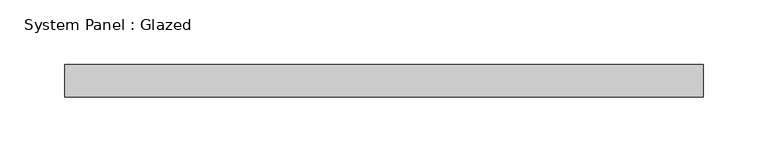
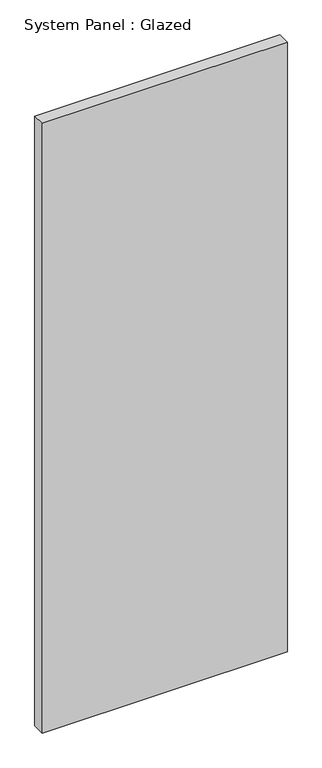
"""IFC4 building model written with IfcOpenShell, lengths in millimetres: plate geometry, System Panel : Glazed."""

from ifc_helpers import new_model, si_unit, origin, origin_with_axes, place, context, project, spatial, polyline, outline, extrude, source, transform, mapped, element, save


def system_panel_glazed_464a4b5e(model_context):
    return source(origin(), model_context, "Body", "SweptSolid", [
        extrude(outline(polyline([(247.65, 19.05), (-247.65, 19.05), (-247.65, 44.45), (247.65, 44.45), (247.65, 19.05)])), origin_with_axes(), (0.0, 0.0, 1.0), 1301.2525568),
    ])


if __name__ == "__main__":
    model = new_model("IFC4")
    model_context = context("Model", 3, world=origin())
    ifc_project = project(units=[si_unit("LENGTHUNIT", "METRE", prefix="MILLI")], contexts=[model_context])
    site = spatial("IfcSite", under=ifc_project)
    building = spatial("IfcBuilding", under=site)
    placement = place(None, origin())
    system_panel_glazed_shape = system_panel_glazed_464a4b5e(model_context)
    element("IfcPlate", 1, ObjectType="System Panel : Glazed", at=placement, inside=building, context=model_context, shape_type="MappedRepresentation", body=[
        mapped(system_panel_glazed_shape, transform((0.0, 0.0, 0.0), x_axis=(1.0, 0.0, 0.0), y_axis=(0.0, 1.0, 0.0), z_axis=(0.0, 0.0, 1.0))),
    ])
    save(model, "model.ifc")

# Revit data of these elements
# Type "System Panel : Glazed"
#   Construction Type Id = "GSP4R"
#   Analytic Construction = "1/8 in Pilkington single glazing"
#   Visual Light Transmittance = 0.9
#   Solar Heat Gain Coefficient = 0.86
#   Heat Transfer Coefficient (U) = 1.18115 BTU/(h·ft²·°F)
#   Define Thermal Properties by = 1
# Element 1 (IfcPlate, "System Panel : Glazed")
#   Materials on its faces: "Glass"
# Materials
#   "Glass": class "Glass", colour RGB 0 128 192, transparency 0.75, Description = "Soda Lime Glass", Cost = 0
